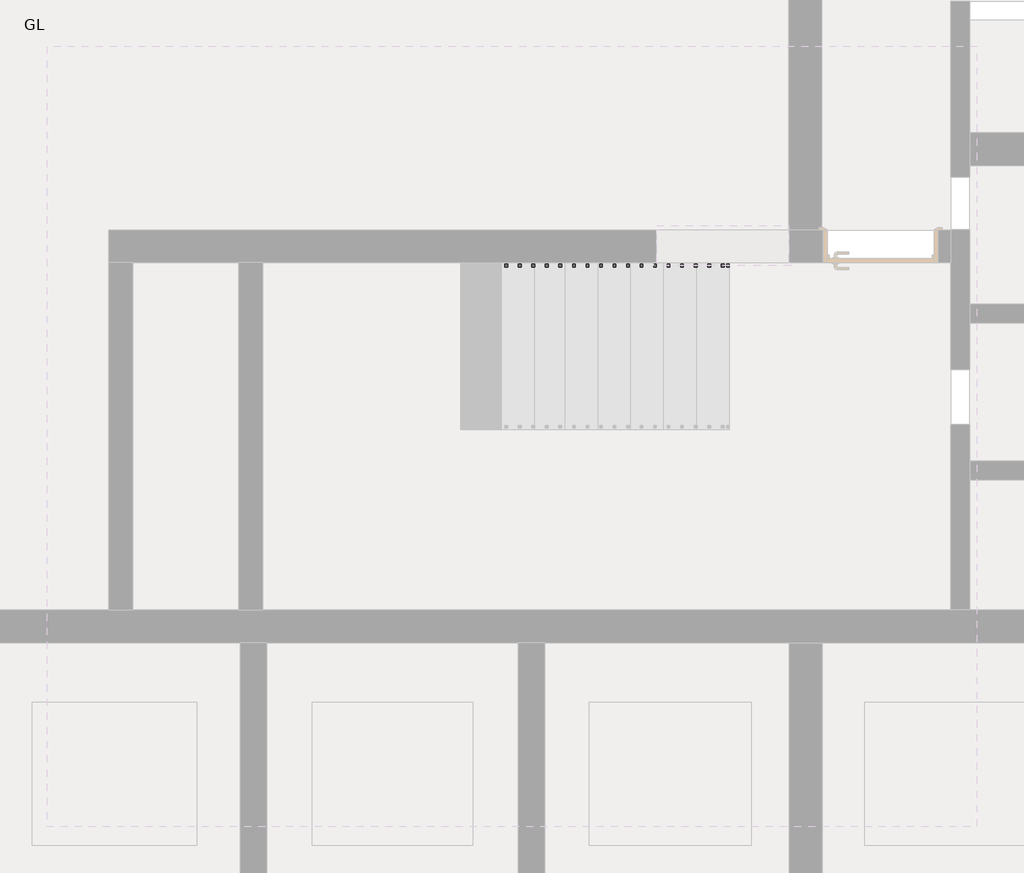
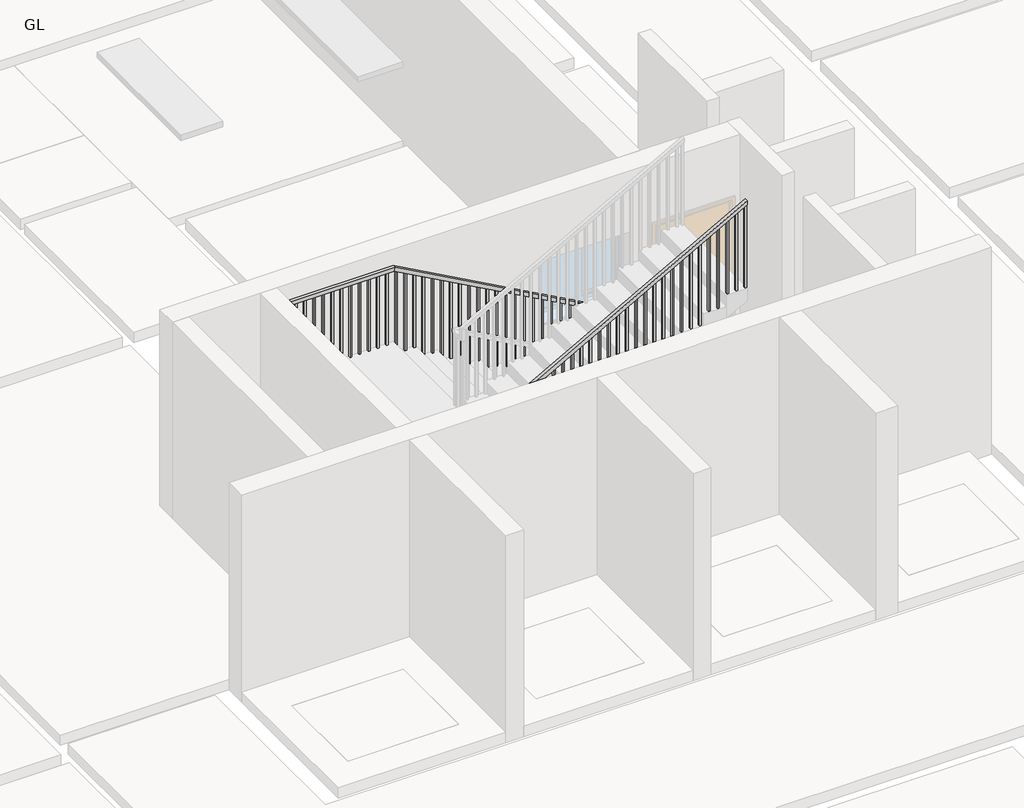
# One storey, part 12 of 14: 1 railing.
"""IFC4 building model written with IfcOpenShell, lengths in millimetres."""

from ifc_helpers import new_model, si_unit, frame, origin, place, context, project, spatial, polyline, outline, extrude, faceted_brep, element, save

model = new_model("IFC4")

# Units and contexts
model_context = context("Model", 3, world=origin())
ifc_project = project(units=[si_unit("LENGTHUNIT", "METRE", prefix="MILLI")], contexts=[model_context])

# Site, building, storey
site = spatial("IfcSite", under=ifc_project)
building = spatial("IfcBuilding", under=site)
storey = spatial("IfcBuildingStorey", under=building, Name="GL", Elevation=0.0)

# Railing
placement = place(None, origin())
element("IfcRailing", 1, ObjectType="1100mm", at=placement, inside=storey, context=model_context, shape_type="SolidModel", body=[
    faceted_brep([(3830.8691495, 82107.3073985, 1266.6666667), (3830.8691495, 82107.3073985, 1209.5255958), (3830.8691495, 82157.3073985, 1209.5255958), (3830.8691495, 82157.3073985, 1266.6666667), (1119.4191495, 82107.3073985, 2766.6666667), (1106.5107118, 82107.3073985, 2716.6666667), (1106.5107118, 82157.3073985, 2716.6666667), (1119.4191495, 82157.3073985, 2766.6666667), (-428.2271613, 82107.3073985, 2766.6666667), (-428.2271613, 82107.3073985, 2716.6666667), (-478.2271613, 82157.3073985, 2716.6666667), (-478.2271613, 82157.3073985, 2766.6666667), (-428.2271613, 78998.7487724, 2766.6666667), (-428.2271613, 78998.7487724, 2716.6666667), (-478.2271613, 78948.7487724, 2716.6666667), (-478.2271613, 78948.7487724, 2766.6666667), (819.4837806, 78998.7487724, 2766.6666667), (832.4425225, 78998.7487724, 2716.6666667), (832.4425225, 78948.7487724, 2716.6666667), (819.4837806, 78948.7487724, 2766.6666667), (4118.7728387, 78998.7487724, 4600.0), (4118.7728387, 78948.7487724, 4600.0), (4118.7728387, 78948.7487724, 4542.7991476), (4118.7728387, 78998.7487724, 4542.7991476)], [[[0, 1, 2, 3]], [[1, 0, 4, 5]], [[2, 1, 5, 6]], [[3, 2, 6, 7]], [[0, 3, 7, 4]], [[5, 4, 8, 9]], [[6, 5, 9, 10]], [[7, 6, 10, 11]], [[4, 7, 11, 8]], [[9, 8, 12, 13]], [[10, 9, 13, 14]], [[11, 10, 14, 15]], [[8, 11, 15, 12]], [[13, 12, 16, 17]], [[14, 13, 17, 18]], [[15, 14, 18, 19]], [[12, 15, 19, 16]], [[20, 21, 22, 23]], [[17, 16, 20, 23]], [[18, 17, 23, 22]], [[19, 18, 22, 21]], [[16, 19, 21, 20]]]),
    extrude(outline(polyline([(4530.5742917, 4096.7728387), (3333.3333333, 4096.7728387), (3333.3333333, 4121.7728387), (4544.4661735, 4121.7728387), (4530.5742917, 4096.7728387)])), frame((0.0, 78961.2487724, 0.0), z_axis=(0.0, 1.0, 0.0), x_axis=(0.0, 0.0, 1.0)), (0.0, 0.0, 1.0), 25.0),
    extrude(outline(polyline([(4461.1148832, 3971.7728387), (3333.3333333, 3971.7728387), (3333.3333333, 3996.7728387), (4475.0067649, 3996.7728387), (4461.1148832, 3971.7728387)])), frame((0.0, 78961.2487724, 0.0), z_axis=(0.0, 1.0, 0.0), x_axis=(0.0, 0.0, 1.0)), (0.0, 0.0, 1.0), 25.0),
    extrude(outline(polyline([(4391.6554746, 3846.7728387), (3333.3333333, 3846.7728387), (3333.3333333, 3871.7728387), (4405.5473563, 3871.7728387), (4391.6554746, 3846.7728387)])), frame((0.0, 78961.2487724, 0.0), z_axis=(0.0, 1.0, 0.0), x_axis=(0.0, 0.0, 1.0)), (0.0, 0.0, 1.0), 25.0),
    extrude(outline(polyline([(4322.196066, 3721.7728387), (3166.6666667, 3721.7728387), (3166.6666667, 3746.7728387), (4336.0879477, 3746.7728387), (4322.196066, 3721.7728387)])), frame((0.0, 78961.2487724, 0.0), z_axis=(0.0, 1.0, 0.0), x_axis=(0.0, 0.0, 1.0)), (0.0, 0.0, 1.0), 25.0),
    extrude(outline(polyline([(4252.7366575, 3596.7728387), (3166.6666667, 3596.7728387), (3166.6666667, 3621.7728387), (4266.6285392, 3621.7728387), (4252.7366575, 3596.7728387)])), frame((0.0, 78961.2487724, 0.0), z_axis=(0.0, 1.0, 0.0), x_axis=(0.0, 0.0, 1.0)), (0.0, 0.0, 1.0), 25.0),
    extrude(outline(polyline([(4183.2772489, 3471.7728387), (3000.0, 3471.7728387), (3000.0, 3496.7728387), (4197.1691306, 3496.7728387), (4183.2772489, 3471.7728387)])), frame((0.0, 78961.2487724, 0.0), z_axis=(0.0, 1.0, 0.0), x_axis=(0.0, 0.0, 1.0)), (0.0, 0.0, 1.0), 25.0),
    extrude(outline(polyline([(4113.8178403, 3346.7728387), (3000.0, 3346.7728387), (3000.0, 3371.7728387), (4127.709722, 3371.7728387), (4113.8178403, 3346.7728387)])), frame((0.0, 78961.2487724, 0.0), z_axis=(0.0, 1.0, 0.0), x_axis=(0.0, 0.0, 1.0)), (0.0, 0.0, 1.0), 25.0),
    extrude(outline(polyline([(4044.3584318, 3221.7728387), (3000.0, 3221.7728387), (3000.0, 3246.7728387), (4058.2503135, 3246.7728387), (4044.3584318, 3221.7728387)])), frame((0.0, 78961.2487724, 0.0), z_axis=(0.0, 1.0, 0.0), x_axis=(0.0, 0.0, 1.0)), (0.0, 0.0, 1.0), 25.0),
    extrude(outline(polyline([(3974.8990232, 3096.7728387), (2833.3333333, 3096.7728387), (2833.3333333, 3121.7728387), (3988.7909049, 3121.7728387), (3974.8990232, 3096.7728387)])), frame((0.0, 78961.2487724, 0.0), z_axis=(0.0, 1.0, 0.0), x_axis=(0.0, 0.0, 1.0)), (0.0, 0.0, 1.0), 25.0),
    extrude(outline(polyline([(3905.4396146, 2971.7728387), (2833.3333333, 2971.7728387), (2833.3333333, 2996.7728387), (3919.3314963, 2996.7728387), (3905.4396146, 2971.7728387)])), frame((0.0, 78961.2487724, 0.0), z_axis=(0.0, 1.0, 0.0), x_axis=(0.0, 0.0, 1.0)), (0.0, 0.0, 1.0), 25.0),
    extrude(outline(polyline([(3835.9802061, 2846.7728387), (2666.6666667, 2846.7728387), (2666.6666667, 2871.7728387), (3849.8720878, 2871.7728387), (3835.9802061, 2846.7728387)])), frame((0.0, 78961.2487724, 0.0), z_axis=(0.0, 1.0, 0.0), x_axis=(0.0, 0.0, 1.0)), (0.0, 0.0, 1.0), 25.0),
    extrude(outline(polyline([(3766.5207975, 2721.7728387), (2666.6666667, 2721.7728387), (2666.6666667, 2746.7728387), (3780.4126792, 2746.7728387), (3766.5207975, 2721.7728387)])), frame((0.0, 78961.2487724, 0.0), z_axis=(0.0, 1.0, 0.0), x_axis=(0.0, 0.0, 1.0)), (0.0, 0.0, 1.0), 25.0),
    extrude(outline(polyline([(3697.0613889, 2596.7728387), (2500.0, 2596.7728387), (2500.0, 2621.7728387), (3710.9532706, 2621.7728387), (3697.0613889, 2596.7728387)])), frame((0.0, 78961.2487724, 0.0), z_axis=(0.0, 1.0, 0.0), x_axis=(0.0, 0.0, 1.0)), (0.0, 0.0, 1.0), 25.0),
    extrude(outline(polyline([(3627.6019804, 2471.7728387), (2500.0, 2471.7728387), (2500.0, 2496.7728387), (3641.4938621, 2496.7728387), (3627.6019804, 2471.7728387)])), frame((0.0, 78961.2487724, 0.0), z_axis=(0.0, 1.0, 0.0), x_axis=(0.0, 0.0, 1.0)), (0.0, 0.0, 1.0), 25.0),
    extrude(outline(polyline([(3558.1425718, 2346.7728387), (2500.0, 2346.7728387), (2500.0, 2371.7728387), (3572.0344535, 2371.7728387), (3558.1425718, 2346.7728387)])), frame((0.0, 78961.2487724, 0.0), z_axis=(0.0, 1.0, 0.0), x_axis=(0.0, 0.0, 1.0)), (0.0, 0.0, 1.0), 25.0),
    extrude(outline(polyline([(3488.6831632, 2221.7728387), (2333.3333333, 2221.7728387), (2333.3333333, 2246.7728387), (3502.5750449, 2246.7728387), (3488.6831632, 2221.7728387)])), frame((0.0, 78961.2487724, 0.0), z_axis=(0.0, 1.0, 0.0), x_axis=(0.0, 0.0, 1.0)), (0.0, 0.0, 1.0), 25.0),
    extrude(outline(polyline([(3419.2237547, 2096.7728387), (2333.3333333, 2096.7728387), (2333.3333333, 2121.7728387), (3433.1156364, 2121.7728387), (3419.2237547, 2096.7728387)])), frame((0.0, 78961.2487724, 0.0), z_axis=(0.0, 1.0, 0.0), x_axis=(0.0, 0.0, 1.0)), (0.0, 0.0, 1.0), 25.0),
    extrude(outline(polyline([(3349.7643461, 1971.7728387), (2166.6666667, 1971.7728387), (2166.6666667, 1996.7728387), (3363.6562278, 1996.7728387), (3349.7643461, 1971.7728387)])), frame((0.0, 78961.2487724, 0.0), z_axis=(0.0, 1.0, 0.0), x_axis=(0.0, 0.0, 1.0)), (0.0, 0.0, 1.0), 25.0),
    extrude(outline(polyline([(3280.3049375, 1846.7728387), (2166.6666667, 1846.7728387), (2166.6666667, 1871.7728387), (3294.1968192, 1871.7728387), (3280.3049375, 1846.7728387)])), frame((0.0, 78961.2487724, 0.0), z_axis=(0.0, 1.0, 0.0), x_axis=(0.0, 0.0, 1.0)), (0.0, 0.0, 1.0), 25.0),
    extrude(outline(polyline([(3210.845529, 1721.7728387), (2166.6666667, 1721.7728387), (2166.6666667, 1746.7728387), (3224.7374107, 1746.7728387), (3210.845529, 1721.7728387)])), frame((0.0, 78961.2487724, 0.0), z_axis=(0.0, 1.0, 0.0), x_axis=(0.0, 0.0, 1.0)), (0.0, 0.0, 1.0), 25.0),
    extrude(outline(polyline([(3141.3861204, 1596.7728387), (2000.0, 1596.7728387), (2000.0, 1621.7728387), (3155.2780021, 1621.7728387), (3141.3861204, 1596.7728387)])), frame((0.0, 78961.2487724, 0.0), z_axis=(0.0, 1.0, 0.0), x_axis=(0.0, 0.0, 1.0)), (0.0, 0.0, 1.0), 25.0),
    extrude(outline(polyline([(3071.9267118, 1471.7728387), (2000.0, 1471.7728387), (2000.0, 1496.7728387), (3085.8185935, 1496.7728387), (3071.9267118, 1471.7728387)])), frame((0.0, 78961.2487724, 0.0), z_axis=(0.0, 1.0, 0.0), x_axis=(0.0, 0.0, 1.0)), (0.0, 0.0, 1.0), 25.0),
    extrude(outline(polyline([(3002.4673033, 1346.7728387), (1833.3333333, 1346.7728387), (1833.3333333, 1371.7728387), (3016.359185, 1371.7728387), (3002.4673033, 1346.7728387)])), frame((0.0, 78961.2487724, 0.0), z_axis=(0.0, 1.0, 0.0), x_axis=(0.0, 0.0, 1.0)), (0.0, 0.0, 1.0), 25.0),
    extrude(outline(polyline([(2933.0078947, 1221.7728387), (1833.3333333, 1221.7728387), (1833.3333333, 1246.7728387), (2946.8997764, 1246.7728387), (2933.0078947, 1221.7728387)])), frame((0.0, 78961.2487724, 0.0), z_axis=(0.0, 1.0, 0.0), x_axis=(0.0, 0.0, 1.0)), (0.0, 0.0, 1.0), 25.0),
    extrude(outline(polyline([(2863.5484861, 1096.7728387), (1666.6666667, 1096.7728387), (1666.6666667, 1121.7728387), (2877.4403678, 1121.7728387), (2863.5484861, 1096.7728387)])), frame((0.0, 78961.2487724, 0.0), z_axis=(0.0, 1.0, 0.0), x_axis=(0.0, 0.0, 1.0)), (0.0, 0.0, 1.0), 25.0),
    extrude(outline(polyline([(2794.0890776, 971.7728387), (1666.6666667, 971.7728387), (1666.6666667, 996.7728387), (2807.9809593, 996.7728387), (2794.0890776, 971.7728387)])), frame((0.0, 78961.2487724, 0.0), z_axis=(0.0, 1.0, 0.0), x_axis=(0.0, 0.0, 1.0)), (0.0, 0.0, 1.0), 25.0),
    extrude(outline(polyline([(2724.629669, 846.7728387), (1666.6666667, 846.7728387), (1666.6666667, 871.7728387), (2738.5215507, 871.7728387), (2724.629669, 846.7728387)])), frame((0.0, 78961.2487724, 0.0), z_axis=(0.0, 1.0, 0.0), x_axis=(0.0, 0.0, 1.0)), (0.0, 0.0, 1.0), 25.0),
    extrude(outline(polyline([(721.7728387, 78961.2487724), (721.7728387, 78986.2487724), (746.7728387, 78986.2487724), (746.7728387, 78961.2487724), (721.7728387, 78961.2487724)])), frame((0.0, 0.0, 1666.6666667), z_axis=(0.0, 0.0, 1.0), x_axis=(1.0, 0.0, 0.0)), (0.0, 0.0, 1.0), 1050.0),
    extrude(outline(polyline([(596.7728387, 78961.2487724), (596.7728387, 78986.2487724), (621.7728387, 78986.2487724), (621.7728387, 78961.2487724), (596.7728387, 78961.2487724)])), frame((0.0, 0.0, 1666.6666667), z_axis=(0.0, 0.0, 1.0), x_axis=(1.0, 0.0, 0.0)), (0.0, 0.0, 1.0), 1050.0),
    extrude(outline(polyline([(471.7728387, 78961.2487724), (471.7728387, 78986.2487724), (496.7728387, 78986.2487724), (496.7728387, 78961.2487724), (471.7728387, 78961.2487724)])), frame((0.0, 0.0, 1666.6666667), z_axis=(0.0, 0.0, 1.0), x_axis=(1.0, 0.0, 0.0)), (0.0, 0.0, 1.0), 1050.0),
    extrude(outline(polyline([(346.7728387, 78961.2487724), (346.7728387, 78986.2487724), (371.7728387, 78986.2487724), (371.7728387, 78961.2487724), (346.7728387, 78961.2487724)])), frame((0.0, 0.0, 1666.6666667), z_axis=(0.0, 0.0, 1.0), x_axis=(1.0, 0.0, 0.0)), (0.0, 0.0, 1.0), 1050.0),
    extrude(outline(polyline([(221.7728387, 78961.2487724), (221.7728387, 78986.2487724), (246.7728387, 78986.2487724), (246.7728387, 78961.2487724), (221.7728387, 78961.2487724)])), frame((0.0, 0.0, 1666.6666667), z_axis=(0.0, 0.0, 1.0), x_axis=(1.0, 0.0, 0.0)), (0.0, 0.0, 1.0), 1050.0),
    extrude(outline(polyline([(96.7728387, 78961.2487724), (96.7728387, 78986.2487724), (121.7728387, 78986.2487724), (121.7728387, 78961.2487724), (96.7728387, 78961.2487724)])), frame((0.0, 0.0, 1666.6666667), z_axis=(0.0, 0.0, 1.0), x_axis=(1.0, 0.0, 0.0)), (0.0, 0.0, 1.0), 1050.0),
    extrude(outline(polyline([(-28.2271613, 78961.2487724), (-28.2271613, 78986.2487724), (-3.2271613, 78986.2487724), (-3.2271613, 78961.2487724), (-28.2271613, 78961.2487724)])), frame((0.0, 0.0, 1666.6666667), z_axis=(0.0, 0.0, 1.0), x_axis=(1.0, 0.0, 0.0)), (0.0, 0.0, 1.0), 1050.0),
    extrude(outline(polyline([(-153.2271613, 78961.2487724), (-153.2271613, 78986.2487724), (-128.2271613, 78986.2487724), (-128.2271613, 78961.2487724), (-153.2271613, 78961.2487724)])), frame((0.0, 0.0, 1666.6666667), z_axis=(0.0, 0.0, 1.0), x_axis=(1.0, 0.0, 0.0)), (0.0, 0.0, 1.0), 1050.0),
    extrude(outline(polyline([(-278.2271613, 78961.2487724), (-278.2271613, 78986.2487724), (-253.2271613, 78986.2487724), (-253.2271613, 78961.2487724), (-278.2271613, 78961.2487724)])), frame((0.0, 0.0, 1666.6666667), z_axis=(0.0, 0.0, 1.0), x_axis=(1.0, 0.0, 0.0)), (0.0, 0.0, 1.0), 1050.0),
    extrude(outline(polyline([(-403.2271613, 78961.2487724), (-403.2271613, 78986.2487724), (-378.2271613, 78986.2487724), (-378.2271613, 78961.2487724), (-403.2271613, 78961.2487724)])), frame((0.0, 0.0, 1666.6666667), z_axis=(0.0, 0.0, 1.0), x_axis=(1.0, 0.0, 0.0)), (0.0, 0.0, 1.0), 1050.0),
    extrude(outline(polyline([(-465.7271613, 79082.3073985), (-440.7271613, 79082.3073985), (-440.7271613, 79057.3073985), (-465.7271613, 79057.3073985), (-465.7271613, 79082.3073985)])), frame((0.0, 0.0, 1666.6666667), z_axis=(0.0, 0.0, 1.0), x_axis=(1.0, 0.0, 0.0)), (0.0, 0.0, 1.0), 1050.0),
    extrude(outline(polyline([(-465.7271613, 79207.3073985), (-440.7271613, 79207.3073985), (-440.7271613, 79182.3073985), (-465.7271613, 79182.3073985), (-465.7271613, 79207.3073985)])), frame((0.0, 0.0, 1666.6666667), z_axis=(0.0, 0.0, 1.0), x_axis=(1.0, 0.0, 0.0)), (0.0, 0.0, 1.0), 1050.0),
    extrude(outline(polyline([(-465.7271613, 79332.3073985), (-440.7271613, 79332.3073985), (-440.7271613, 79307.3073985), (-465.7271613, 79307.3073985), (-465.7271613, 79332.3073985)])), frame((0.0, 0.0, 1666.6666667), z_axis=(0.0, 0.0, 1.0), x_axis=(1.0, 0.0, 0.0)), (0.0, 0.0, 1.0), 1050.0),
    extrude(outline(polyline([(-465.7271613, 79457.3073985), (-440.7271613, 79457.3073985), (-440.7271613, 79432.3073985), (-465.7271613, 79432.3073985), (-465.7271613, 79457.3073985)])), frame((0.0, 0.0, 1666.6666667), z_axis=(0.0, 0.0, 1.0), x_axis=(1.0, 0.0, 0.0)), (0.0, 0.0, 1.0), 1050.0),
    extrude(outline(polyline([(-465.7271613, 79582.3073985), (-440.7271613, 79582.3073985), (-440.7271613, 79557.3073985), (-465.7271613, 79557.3073985), (-465.7271613, 79582.3073985)])), frame((0.0, 0.0, 1666.6666667), z_axis=(0.0, 0.0, 1.0), x_axis=(1.0, 0.0, 0.0)), (0.0, 0.0, 1.0), 1050.0),
    extrude(outline(polyline([(-465.7271613, 79707.3073985), (-440.7271613, 79707.3073985), (-440.7271613, 79682.3073985), (-465.7271613, 79682.3073985), (-465.7271613, 79707.3073985)])), frame((0.0, 0.0, 1666.6666667), z_axis=(0.0, 0.0, 1.0), x_axis=(1.0, 0.0, 0.0)), (0.0, 0.0, 1.0), 1050.0),
    extrude(outline(polyline([(-465.7271613, 79832.3073985), (-440.7271613, 79832.3073985), (-440.7271613, 79807.3073985), (-465.7271613, 79807.3073985), (-465.7271613, 79832.3073985)])), frame((0.0, 0.0, 1666.6666667), z_axis=(0.0, 0.0, 1.0), x_axis=(1.0, 0.0, 0.0)), (0.0, 0.0, 1.0), 1050.0),
    extrude(outline(polyline([(-465.7271613, 79957.3073985), (-440.7271613, 79957.3073985), (-440.7271613, 79932.3073985), (-465.7271613, 79932.3073985), (-465.7271613, 79957.3073985)])), frame((0.0, 0.0, 1666.6666667), z_axis=(0.0, 0.0, 1.0), x_axis=(1.0, 0.0, 0.0)), (0.0, 0.0, 1.0), 1050.0),
    extrude(outline(polyline([(-465.7271613, 80082.3073985), (-440.7271613, 80082.3073985), (-440.7271613, 80057.3073985), (-465.7271613, 80057.3073985), (-465.7271613, 80082.3073985)])), frame((0.0, 0.0, 1666.6666667), z_axis=(0.0, 0.0, 1.0), x_axis=(1.0, 0.0, 0.0)), (0.0, 0.0, 1.0), 1050.0),
    extrude(outline(polyline([(-465.7271613, 80207.3073985), (-440.7271613, 80207.3073985), (-440.7271613, 80182.3073985), (-465.7271613, 80182.3073985), (-465.7271613, 80207.3073985)])), frame((0.0, 0.0, 1666.6666667), z_axis=(0.0, 0.0, 1.0), x_axis=(1.0, 0.0, 0.0)), (0.0, 0.0, 1.0), 1050.0),
    extrude(outline(polyline([(-465.7271613, 80332.3073985), (-440.7271613, 80332.3073985), (-440.7271613, 80307.3073985), (-465.7271613, 80307.3073985), (-465.7271613, 80332.3073985)])), frame((0.0, 0.0, 1666.6666667), z_axis=(0.0, 0.0, 1.0), x_axis=(1.0, 0.0, 0.0)), (0.0, 0.0, 1.0), 1050.0),
    extrude(outline(polyline([(-465.7271613, 80457.3073985), (-440.7271613, 80457.3073985), (-440.7271613, 80432.3073985), (-465.7271613, 80432.3073985), (-465.7271613, 80457.3073985)])), frame((0.0, 0.0, 1666.6666667), z_axis=(0.0, 0.0, 1.0), x_axis=(1.0, 0.0, 0.0)), (0.0, 0.0, 1.0), 1050.0),
    extrude(outline(polyline([(-465.7271613, 80582.3073985), (-440.7271613, 80582.3073985), (-440.7271613, 80557.3073985), (-465.7271613, 80557.3073985), (-465.7271613, 80582.3073985)])), frame((0.0, 0.0, 1666.6666667), z_axis=(0.0, 0.0, 1.0), x_axis=(1.0, 0.0, 0.0)), (0.0, 0.0, 1.0), 1050.0),
    extrude(outline(polyline([(-465.7271613, 80707.3073985), (-440.7271613, 80707.3073985), (-440.7271613, 80682.3073985), (-465.7271613, 80682.3073985), (-465.7271613, 80707.3073985)])), frame((0.0, 0.0, 1666.6666667), z_axis=(0.0, 0.0, 1.0), x_axis=(1.0, 0.0, 0.0)), (0.0, 0.0, 1.0), 1050.0),
    extrude(outline(polyline([(-465.7271613, 80832.3073985), (-440.7271613, 80832.3073985), (-440.7271613, 80807.3073985), (-465.7271613, 80807.3073985), (-465.7271613, 80832.3073985)])), frame((0.0, 0.0, 1666.6666667), z_axis=(0.0, 0.0, 1.0), x_axis=(1.0, 0.0, 0.0)), (0.0, 0.0, 1.0), 1050.0),
    extrude(outline(polyline([(-465.7271613, 80957.3073985), (-440.7271613, 80957.3073985), (-440.7271613, 80932.3073985), (-465.7271613, 80932.3073985), (-465.7271613, 80957.3073985)])), frame((0.0, 0.0, 1666.6666667), z_axis=(0.0, 0.0, 1.0), x_axis=(1.0, 0.0, 0.0)), (0.0, 0.0, 1.0), 1050.0),
    extrude(outline(polyline([(-465.7271613, 81082.3073985), (-440.7271613, 81082.3073985), (-440.7271613, 81057.3073985), (-465.7271613, 81057.3073985), (-465.7271613, 81082.3073985)])), frame((0.0, 0.0, 1666.6666667), z_axis=(0.0, 0.0, 1.0), x_axis=(1.0, 0.0, 0.0)), (0.0, 0.0, 1.0), 1050.0),
    extrude(outline(polyline([(-465.7271613, 81207.3073985), (-440.7271613, 81207.3073985), (-440.7271613, 81182.3073985), (-465.7271613, 81182.3073985), (-465.7271613, 81207.3073985)])), frame((0.0, 0.0, 1666.6666667), z_axis=(0.0, 0.0, 1.0), x_axis=(1.0, 0.0, 0.0)), (0.0, 0.0, 1.0), 1050.0),
    extrude(outline(polyline([(-465.7271613, 81332.3073985), (-440.7271613, 81332.3073985), (-440.7271613, 81307.3073985), (-465.7271613, 81307.3073985), (-465.7271613, 81332.3073985)])), frame((0.0, 0.0, 1666.6666667), z_axis=(0.0, 0.0, 1.0), x_axis=(1.0, 0.0, 0.0)), (0.0, 0.0, 1.0), 1050.0),
    extrude(outline(polyline([(-465.7271613, 81457.3073985), (-440.7271613, 81457.3073985), (-440.7271613, 81432.3073985), (-465.7271613, 81432.3073985), (-465.7271613, 81457.3073985)])), frame((0.0, 0.0, 1666.6666667), z_axis=(0.0, 0.0, 1.0), x_axis=(1.0, 0.0, 0.0)), (0.0, 0.0, 1.0), 1050.0),
    extrude(outline(polyline([(-465.7271613, 81582.3073985), (-440.7271613, 81582.3073985), (-440.7271613, 81557.3073985), (-465.7271613, 81557.3073985), (-465.7271613, 81582.3073985)])), frame((0.0, 0.0, 1666.6666667), z_axis=(0.0, 0.0, 1.0), x_axis=(1.0, 0.0, 0.0)), (0.0, 0.0, 1.0), 1050.0),
    extrude(outline(polyline([(-465.7271613, 81707.3073985), (-440.7271613, 81707.3073985), (-440.7271613, 81682.3073985), (-465.7271613, 81682.3073985), (-465.7271613, 81707.3073985)])), frame((0.0, 0.0, 1666.6666667), z_axis=(0.0, 0.0, 1.0), x_axis=(1.0, 0.0, 0.0)), (0.0, 0.0, 1.0), 1050.0),
    extrude(outline(polyline([(-465.7271613, 81832.3073985), (-440.7271613, 81832.3073985), (-440.7271613, 81807.3073985), (-465.7271613, 81807.3073985), (-465.7271613, 81832.3073985)])), frame((0.0, 0.0, 1666.6666667), z_axis=(0.0, 0.0, 1.0), x_axis=(1.0, 0.0, 0.0)), (0.0, 0.0, 1.0), 1050.0),
    extrude(outline(polyline([(-465.7271613, 81957.3073985), (-440.7271613, 81957.3073985), (-440.7271613, 81932.3073985), (-465.7271613, 81932.3073985), (-465.7271613, 81957.3073985)])), frame((0.0, 0.0, 1666.6666667), z_axis=(0.0, 0.0, 1.0), x_axis=(1.0, 0.0, 0.0)), (0.0, 0.0, 1.0), 1050.0),
    extrude(outline(polyline([(-465.7271613, 82082.3073985), (-440.7271613, 82082.3073985), (-440.7271613, 82057.3073985), (-465.7271613, 82057.3073985), (-465.7271613, 82082.3073985)])), frame((0.0, 0.0, 1666.6666667), z_axis=(0.0, 0.0, 1.0), x_axis=(1.0, 0.0, 0.0)), (0.0, 0.0, 1.0), 1050.0),
    extrude(outline(polyline([(-344.1308505, 82144.8073985), (-344.1308505, 82119.8073985), (-369.1308505, 82119.8073985), (-369.1308505, 82144.8073985), (-344.1308505, 82144.8073985)])), frame((0.0, 0.0, 1666.6666667), z_axis=(0.0, 0.0, 1.0), x_axis=(1.0, 0.0, 0.0)), (0.0, 0.0, 1.0), 1050.0),
    extrude(outline(polyline([(-219.1308505, 82144.8073985), (-219.1308505, 82119.8073985), (-244.1308505, 82119.8073985), (-244.1308505, 82144.8073985), (-219.1308505, 82144.8073985)])), frame((0.0, 0.0, 1666.6666667), z_axis=(0.0, 0.0, 1.0), x_axis=(1.0, 0.0, 0.0)), (0.0, 0.0, 1.0), 1050.0),
    extrude(outline(polyline([(-94.1308505, 82144.8073985), (-94.1308505, 82119.8073985), (-119.1308505, 82119.8073985), (-119.1308505, 82144.8073985), (-94.1308505, 82144.8073985)])), frame((0.0, 0.0, 1666.6666667), z_axis=(0.0, 0.0, 1.0), x_axis=(1.0, 0.0, 0.0)), (0.0, 0.0, 1.0), 1050.0),
    extrude(outline(polyline([(30.8691495, 82144.8073985), (30.8691495, 82119.8073985), (5.8691495, 82119.8073985), (5.8691495, 82144.8073985), (30.8691495, 82144.8073985)])), frame((0.0, 0.0, 1666.6666667), z_axis=(0.0, 0.0, 1.0), x_axis=(1.0, 0.0, 0.0)), (0.0, 0.0, 1.0), 1050.0),
    extrude(outline(polyline([(155.8691495, 82144.8073985), (155.8691495, 82119.8073985), (130.8691495, 82119.8073985), (130.8691495, 82144.8073985), (155.8691495, 82144.8073985)])), frame((0.0, 0.0, 1666.6666667), z_axis=(0.0, 0.0, 1.0), x_axis=(1.0, 0.0, 0.0)), (0.0, 0.0, 1.0), 1050.0),
    extrude(outline(polyline([(280.8691495, 82144.8073985), (280.8691495, 82119.8073985), (255.8691495, 82119.8073985), (255.8691495, 82144.8073985), (280.8691495, 82144.8073985)])), frame((0.0, 0.0, 1666.6666667), z_axis=(0.0, 0.0, 1.0), x_axis=(1.0, 0.0, 0.0)), (0.0, 0.0, 1.0), 1050.0),
    extrude(outline(polyline([(405.8691495, 82144.8073985), (405.8691495, 82119.8073985), (380.8691495, 82119.8073985), (380.8691495, 82144.8073985), (405.8691495, 82144.8073985)])), frame((0.0, 0.0, 1666.6666667), z_axis=(0.0, 0.0, 1.0), x_axis=(1.0, 0.0, 0.0)), (0.0, 0.0, 1.0), 1050.0),
    extrude(outline(polyline([(530.8691495, 82144.8073985), (530.8691495, 82119.8073985), (505.8691495, 82119.8073985), (505.8691495, 82144.8073985), (530.8691495, 82144.8073985)])), frame((0.0, 0.0, 1666.6666667), z_axis=(0.0, 0.0, 1.0), x_axis=(1.0, 0.0, 0.0)), (0.0, 0.0, 1.0), 1050.0),
    extrude(outline(polyline([(655.8691495, 82144.8073985), (655.8691495, 82119.8073985), (630.8691495, 82119.8073985), (630.8691495, 82144.8073985), (655.8691495, 82144.8073985)])), frame((0.0, 0.0, 1666.6666667), z_axis=(0.0, 0.0, 1.0), x_axis=(1.0, 0.0, 0.0)), (0.0, 0.0, 1.0), 1050.0),
    extrude(outline(polyline([(780.8691495, 82144.8073985), (780.8691495, 82119.8073985), (755.8691495, 82119.8073985), (755.8691495, 82144.8073985), (780.8691495, 82144.8073985)])), frame((0.0, 0.0, 1666.6666667), z_axis=(0.0, 0.0, 1.0), x_axis=(1.0, 0.0, 0.0)), (0.0, 0.0, 1.0), 1050.0),
    extrude(outline(polyline([(905.8691495, 82144.8073985), (905.8691495, 82119.8073985), (880.8691495, 82119.8073985), (880.8691495, 82144.8073985), (905.8691495, 82144.8073985)])), frame((0.0, 0.0, 1666.6666667), z_axis=(0.0, 0.0, 1.0), x_axis=(1.0, 0.0, 0.0)), (0.0, 0.0, 1.0), 1050.0),
    extrude(outline(polyline([(1030.8691495, 82144.8073985), (1030.8691495, 82119.8073985), (1005.8691495, 82119.8073985), (1005.8691495, 82144.8073985), (1030.8691495, 82144.8073985)])), frame((0.0, 0.0, 1666.6666667), z_axis=(0.0, 0.0, 1.0), x_axis=(1.0, 0.0, 0.0)), (0.0, 0.0, 1.0), 1050.0),
    extrude(outline(polyline([(1500.0, 1155.8691495), (2689.3611082, 1155.8691495), (2703.1913466, 1130.8691495), (1500.0, 1130.8691495), (1500.0, 1155.8691495)])), frame((0.0, 82119.8073985, 0.0), z_axis=(0.0, 1.0, 0.0), x_axis=(0.0, 0.0, 1.0)), (0.0, 0.0, 1.0), 25.0),
    extrude(outline(polyline([(1500.0, 1280.8691495), (2620.209916, 1280.8691495), (2634.0401544, 1255.8691495), (1500.0, 1255.8691495), (1500.0, 1280.8691495)])), frame((0.0, 82119.8073985, 0.0), z_axis=(0.0, 1.0, 0.0), x_axis=(0.0, 0.0, 1.0)), (0.0, 0.0, 1.0), 25.0),
    extrude(outline(polyline([(1500.0, 1405.8691495), (2551.0587238, 1405.8691495), (2564.8889623, 1380.8691495), (1500.0, 1380.8691495), (1500.0, 1405.8691495)])), frame((0.0, 82119.8073985, 0.0), z_axis=(0.0, 1.0, 0.0), x_axis=(0.0, 0.0, 1.0)), (0.0, 0.0, 1.0), 25.0),
    extrude(outline(polyline([(1333.3333333, 1530.8691495), (2481.9075317, 1530.8691495), (2495.7377701, 1505.8691495), (1333.3333333, 1505.8691495), (1333.3333333, 1530.8691495)])), frame((0.0, 82119.8073985, 0.0), z_axis=(0.0, 1.0, 0.0), x_axis=(0.0, 0.0, 1.0)), (0.0, 0.0, 1.0), 25.0),
    extrude(outline(polyline([(1333.3333333, 1655.8691495), (2412.7563395, 1655.8691495), (2426.5865779, 1630.8691495), (1333.3333333, 1630.8691495), (1333.3333333, 1655.8691495)])), frame((0.0, 82119.8073985, 0.0), z_axis=(0.0, 1.0, 0.0), x_axis=(0.0, 0.0, 1.0)), (0.0, 0.0, 1.0), 25.0),
    extrude(outline(polyline([(1166.6666667, 1780.8691495), (2343.6051473, 1780.8691495), (2357.4353858, 1755.8691495), (1166.6666667, 1755.8691495), (1166.6666667, 1780.8691495)])), frame((0.0, 82119.8073985, 0.0), z_axis=(0.0, 1.0, 0.0), x_axis=(0.0, 0.0, 1.0)), (0.0, 0.0, 1.0), 25.0),
    extrude(outline(polyline([(1166.6666667, 1905.8691495), (2274.4539552, 1905.8691495), (2288.2841936, 1880.8691495), (1166.6666667, 1880.8691495), (1166.6666667, 1905.8691495)])), frame((0.0, 82119.8073985, 0.0), z_axis=(0.0, 1.0, 0.0), x_axis=(0.0, 0.0, 1.0)), (0.0, 0.0, 1.0), 25.0),
    extrude(outline(polyline([(1166.6666667, 2030.8691495), (2205.302763, 2030.8691495), (2219.1330014, 2005.8691495), (1166.6666667, 2005.8691495), (1166.6666667, 2030.8691495)])), frame((0.0, 82119.8073985, 0.0), z_axis=(0.0, 1.0, 0.0), x_axis=(0.0, 0.0, 1.0)), (0.0, 0.0, 1.0), 25.0),
    extrude(outline(polyline([(1000.0, 2155.8691495), (2136.1515708, 2155.8691495), (2149.9818093, 2130.8691495), (1000.0, 2130.8691495), (1000.0, 2155.8691495)])), frame((0.0, 82119.8073985, 0.0), z_axis=(0.0, 1.0, 0.0), x_axis=(0.0, 0.0, 1.0)), (0.0, 0.0, 1.0), 25.0),
    extrude(outline(polyline([(1000.0, 2280.8691495), (2067.0003787, 2280.8691495), (2080.8306171, 2255.8691495), (1000.0, 2255.8691495), (1000.0, 2280.8691495)])), frame((0.0, 82119.8073985, 0.0), z_axis=(0.0, 1.0, 0.0), x_axis=(0.0, 0.0, 1.0)), (0.0, 0.0, 1.0), 25.0),
    extrude(outline(polyline([(833.3333333, 2405.8691495), (1997.8491865, 2405.8691495), (2011.6794249, 2380.8691495), (833.3333333, 2380.8691495), (833.3333333, 2405.8691495)])), frame((0.0, 82119.8073985, 0.0), z_axis=(0.0, 1.0, 0.0), x_axis=(0.0, 0.0, 1.0)), (0.0, 0.0, 1.0), 25.0),
    extrude(outline(polyline([(833.3333333, 2530.8691495), (1928.6979943, 2530.8691495), (1942.5282328, 2505.8691495), (833.3333333, 2505.8691495), (833.3333333, 2530.8691495)])), frame((0.0, 82119.8073985, 0.0), z_axis=(0.0, 1.0, 0.0), x_axis=(0.0, 0.0, 1.0)), (0.0, 0.0, 1.0), 25.0),
    extrude(outline(polyline([(666.6666667, 2655.8691495), (1859.5468022, 2655.8691495), (1873.3770406, 2630.8691495), (666.6666667, 2630.8691495), (666.6666667, 2655.8691495)])), frame((0.0, 82119.8073985, 0.0), z_axis=(0.0, 1.0, 0.0), x_axis=(0.0, 0.0, 1.0)), (0.0, 0.0, 1.0), 25.0),
    extrude(outline(polyline([(666.6666667, 2780.8691495), (1790.39561, 2780.8691495), (1804.2258484, 2755.8691495), (666.6666667, 2755.8691495), (666.6666667, 2780.8691495)])), frame((0.0, 82119.8073985, 0.0), z_axis=(0.0, 1.0, 0.0), x_axis=(0.0, 0.0, 1.0)), (0.0, 0.0, 1.0), 25.0),
    extrude(outline(polyline([(666.6666667, 2905.8691495), (1721.2444178, 2905.8691495), (1735.0746563, 2880.8691495), (666.6666667, 2880.8691495), (666.6666667, 2905.8691495)])), frame((0.0, 82119.8073985, 0.0), z_axis=(0.0, 1.0, 0.0), x_axis=(0.0, 0.0, 1.0)), (0.0, 0.0, 1.0), 25.0),
    extrude(outline(polyline([(500.0, 3030.8691495), (1652.0932257, 3030.8691495), (1665.9234641, 3005.8691495), (500.0, 3005.8691495), (500.0, 3030.8691495)])), frame((0.0, 82119.8073985, 0.0), z_axis=(0.0, 1.0, 0.0), x_axis=(0.0, 0.0, 1.0)), (0.0, 0.0, 1.0), 25.0),
    extrude(outline(polyline([(500.0, 3155.8691495), (1582.9420335, 3155.8691495), (1596.7722719, 3130.8691495), (500.0, 3130.8691495), (500.0, 3155.8691495)])), frame((0.0, 82119.8073985, 0.0), z_axis=(0.0, 1.0, 0.0), x_axis=(0.0, 0.0, 1.0)), (0.0, 0.0, 1.0), 25.0),
    extrude(outline(polyline([(333.3333333, 3280.8691495), (1513.7908413, 3280.8691495), (1527.6210798, 3255.8691495), (333.3333333, 3255.8691495), (333.3333333, 3280.8691495)])), frame((0.0, 82119.8073985, 0.0), z_axis=(0.0, 1.0, 0.0), x_axis=(0.0, 0.0, 1.0)), (0.0, 0.0, 1.0), 25.0),
    extrude(outline(polyline([(333.3333333, 3405.8691495), (1444.6396492, 3405.8691495), (1458.4698876, 3380.8691495), (333.3333333, 3380.8691495), (333.3333333, 3405.8691495)])), frame((0.0, 82119.8073985, 0.0), z_axis=(0.0, 1.0, 0.0), x_axis=(0.0, 0.0, 1.0)), (0.0, 0.0, 1.0), 25.0),
    extrude(outline(polyline([(333.3333333, 3530.8691495), (1375.488457, 3530.8691495), (1389.3186954, 3505.8691495), (333.3333333, 3505.8691495), (333.3333333, 3530.8691495)])), frame((0.0, 82119.8073985, 0.0), z_axis=(0.0, 1.0, 0.0), x_axis=(0.0, 0.0, 1.0)), (0.0, 0.0, 1.0), 25.0),
    extrude(outline(polyline([(166.6666667, 3655.8691495), (1306.3372648, 3655.8691495), (1320.1675033, 3630.8691495), (166.6666667, 3630.8691495), (166.6666667, 3655.8691495)])), frame((0.0, 82119.8073985, 0.0), z_axis=(0.0, 1.0, 0.0), x_axis=(0.0, 0.0, 1.0)), (0.0, 0.0, 1.0), 25.0),
    extrude(outline(polyline([(166.6666667, 3780.8691495), (1237.1860727, 3780.8691495), (1251.0163111, 3755.8691495), (166.6666667, 3755.8691495), (166.6666667, 3780.8691495)])), frame((0.0, 82119.8073985, 0.0), z_axis=(0.0, 1.0, 0.0), x_axis=(0.0, 0.0, 1.0)), (0.0, 0.0, 1.0), 25.0),
    extrude(outline(polyline([(-465.7271613, 78986.2487724), (-440.7271613, 78986.2487724), (-440.7271613, 78961.2487724), (-465.7271613, 78961.2487724), (-465.7271613, 78986.2487724)])), frame((0.0, 0.0, 1666.6666667), z_axis=(0.0, 0.0, 1.0), x_axis=(1.0, 0.0, 0.0)), (0.0, 0.0, 1.0), 1050.0),
    extrude(outline(polyline([(-440.7271613, 82144.8073985), (-440.7271613, 82119.8073985), (-465.7271613, 82119.8073985), (-465.7271613, 82144.8073985), (-440.7271613, 82144.8073985)])), frame((0.0, 0.0, 1666.6666667), z_axis=(0.0, 0.0, 1.0), x_axis=(1.0, 0.0, 0.0)), (0.0, 0.0, 1.0), 1050.0),
    extrude(outline(polyline([(4528.9072659, 4093.7728387), (3333.3333333, 4093.7728387), (3333.3333333, 4118.7728387), (4542.7991476, 4118.7728387), (4528.9072659, 4093.7728387)])), frame((0.0, 78961.2487724, 0.0), z_axis=(0.0, 1.0, 0.0), x_axis=(0.0, 0.0, 1.0)), (0.0, 0.0, 1.0), 25.0),
    extrude(outline(polyline([(166.6666667, 3830.8691495), (1209.5255958, 3830.8691495), (1223.3558342, 3805.8691495), (166.6666667, 3805.8691495), (166.6666667, 3830.8691495)])), frame((0.0, 82119.8073985, 0.0), z_axis=(0.0, 1.0, 0.0), x_axis=(0.0, 0.0, 1.0)), (0.0, 0.0, 1.0), 25.0),
])

save(model, "model.ifc")

# Revit data of these elements
# Type "1100mm"
#   built-in parameter 1008612 = 0.019685 (stored number, unit not read)
#   built-in parameter 1008611 = 0.019685 (stored number, unit not read)
#   built-in parameter 1008609 = 0.902231 (stored number, unit not read)
#   built-in parameter 1008604 = 0.19685 (stored number, unit not read)
#   built-in parameter 1008603 = 0.164042 (stored number, unit not read)
#   Railing Height = 3.608924 ft
#   built-in parameter 1008630 = 2
#   built-in parameter 1008610 = 2
#   built-in parameter 1008608 = 1
#   built-in parameter 1008618 = Baluster_Square : 25mm
# Element 1 (IfcRailing, "1100mm")
#   Phase Created = New Construction
